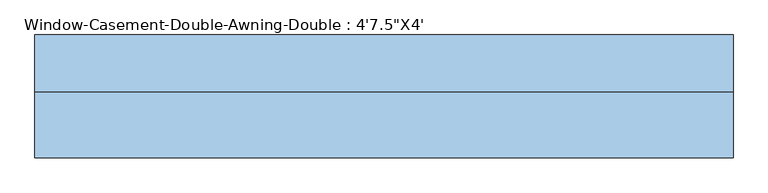
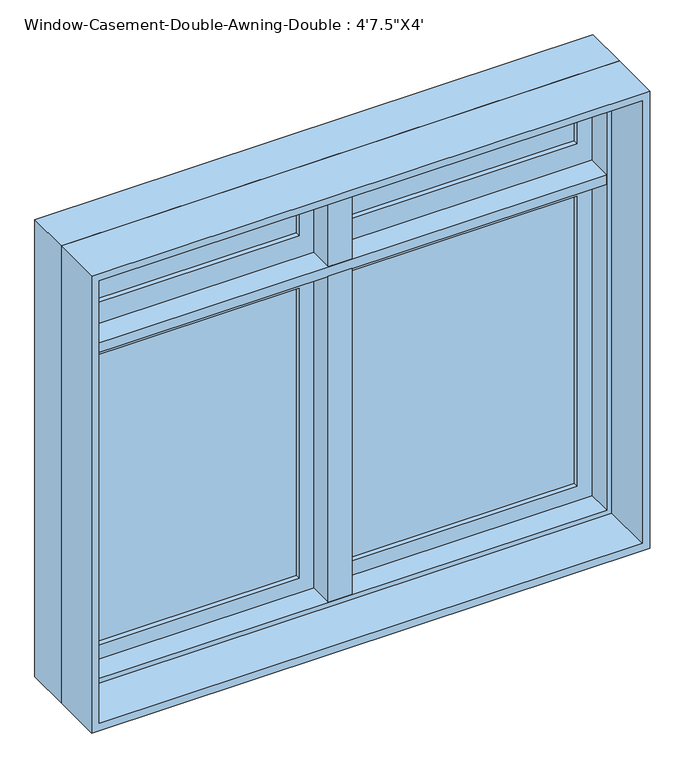
"""IFC4 building model written with IfcOpenShell, lengths in millimetres: window geometry."""

from ifc_helpers import new_model, si_unit, frame, origin, place, context, project, spatial, polyline, outline, extrude, faceted_brep, source, transform, mapped, element, save


def window_c5cb33f6(model_context):
    return source(origin(), model_context, "Body", "SolidModel", [
        faceted_brep([(673.1, 82.55, 2101.85), (673.1, 19.05, 2101.85), (-673.1, 19.05, 2101.85), (-673.1, 82.55, 2101.85), (692.15, 133.35, 2120.9), (692.15, 82.55, 2120.9), (-692.15, 82.55, 2120.9), (-692.15, 133.35, 2120.9), (704.85, 19.05, 2133.6), (704.85, 133.35, 2133.6), (-704.85, 133.35, 2133.6), (-704.85, 19.05, 2133.6), (-673.1, 19.05, 946.15), (-673.1, 82.55, 946.15), (-692.15, 82.55, 927.1), (-692.15, 133.35, 927.1), (-704.85, 133.35, 914.4), (-704.85, 19.05, 914.4), (673.1, 19.05, 946.15), (673.1, 82.55, 946.15), (692.15, 82.55, 927.1), (692.15, 133.35, 927.1), (704.85, 133.35, 914.4), (704.85, 19.05, 914.4)], [[[0, 1, 2, 3]], [[4, 5, 6, 7]], [[8, 9, 10, 11]], [[3, 2, 12, 13]], [[7, 6, 14, 15]], [[11, 10, 16, 17]], [[13, 12, 18, 19]], [[15, 14, 20, 21]], [[17, 16, 22, 23]], [[11, 17, 23, 8], [1, 18, 12, 2]], [[19, 18, 1, 0]], [[5, 20, 14, 6], [3, 13, 19, 0]], [[21, 20, 5, 4]], [[23, 22, 9, 8]], [[9, 22, 16, 10], [7, 15, 21, 4]]]),
        extrude(outline(polyline([(2133.6, -704.85), (914.4, -704.85), (914.4, 704.85), (2133.6, 704.85), (2133.6, -704.85)]), holes=[polyline([(2114.55, 685.8), (933.45, 685.8), (933.45, -685.8), (2114.55, -685.8), (2114.55, 685.8)])]), frame((0.0, -114.3, 0.0), z_axis=(0.0, 1.0, 0.0), x_axis=(0.0, 0.0, 1.0)), (0.0, 0.0, 1.0), 133.35),
        extrude(outline(polyline([(927.1, 692.15), (1816.1, 692.15), (1816.1, 9.525), (927.1, 9.525), (927.1, 692.15)]), holes=[polyline([(984.25, 66.675), (1758.95, 66.675), (1758.95, 635.0), (984.25, 635.0), (984.25, 66.675)])]), frame((0.0, 82.55, 0.0), z_axis=(0.0, 1.0, 0.0), x_axis=(0.0, 0.0, 1.0)), (0.0, 0.0, 1.0), 44.45),
        extrude(outline(polyline([(1816.1, -692.15), (927.1, -692.15), (927.1, -9.525), (1816.1, -9.525), (1816.1, -692.15)]), holes=[polyline([(1758.95, -66.675), (984.25, -66.675), (984.25, -635.0), (1758.95, -635.0), (1758.95, -66.675)])]), frame((0.0, 82.55, 0.0), z_axis=(0.0, 1.0, 0.0), x_axis=(0.0, 0.0, 1.0)), (0.0, 0.0, 1.0), 44.45),
        extrude(outline(polyline([(635.0, 114.3), (635.0, 107.95), (66.675, 107.95), (66.675, 114.3), (635.0, 114.3)])), frame((0.0, 0.0, 984.25), z_axis=(0.0, 0.0, 1.0), x_axis=(1.0, 0.0, 0.0)), (0.0, 0.0, 1.0), 774.7),
        extrude(outline(polyline([(66.675, 95.25), (66.675, 101.6), (635.0, 101.6), (635.0, 95.25), (66.675, 95.25)])), frame((0.0, 0.0, 984.25), z_axis=(0.0, 0.0, 1.0), x_axis=(1.0, 0.0, 0.0)), (0.0, 0.0, 1.0), 774.7),
        extrude(outline(polyline([(-66.675, 114.3), (-66.675, 107.95), (-635.0, 107.95), (-635.0, 114.3), (-66.675, 114.3)])), frame((0.0, 0.0, 984.25), z_axis=(0.0, 0.0, 1.0), x_axis=(1.0, 0.0, 0.0)), (0.0, 0.0, 1.0), 774.7),
        extrude(outline(polyline([(-635.0, 95.25), (-635.0, 101.6), (-66.675, 101.6), (-66.675, 95.25), (-635.0, 95.25)])), frame((0.0, 0.0, 984.25), z_axis=(0.0, 0.0, 1.0), x_axis=(1.0, 0.0, 0.0)), (0.0, 0.0, 1.0), 774.7),
        faceted_brep([(9.525, 133.35, 1816.1), (-9.525, 133.35, 1816.1), (-9.525, 82.55, 1816.1), (-30.1625, 82.55, 1816.1), (-30.1625, 19.05, 1816.1), (30.1625, 19.05, 1816.1), (30.1625, 82.55, 1816.1), (9.525, 82.55, 1816.1), (9.525, 133.35, 927.1), (9.525, 82.55, 927.1), (-9.525, 82.55, 927.1), (-9.525, 133.35, 927.1), (-9.525, 82.55, 946.15), (-30.1625, 82.55, 946.15), (-30.1625, 19.05, 946.15), (30.1625, 19.05, 946.15), (30.1625, 82.55, 946.15), (9.525, 82.55, 946.15)], [[[0, 1, 2, 3, 4, 5, 6, 7]], [[8, 9, 10, 11]], [[1, 0, 8, 11]], [[2, 1, 11, 10, 12]], [[3, 2, 12, 13]], [[4, 3, 13, 14]], [[5, 4, 14, 15]], [[6, 5, 15, 16]], [[7, 6, 16, 17]], [[0, 7, 17, 9, 8]], [[17, 12, 10, 9]], [[12, 17, 16, 15, 14, 13]]]),
        extrude(outline(polyline([(-66.675, 114.3), (-66.675, 107.95), (-635.0, 107.95), (-635.0, 114.3), (-66.675, 114.3)])), frame((0.0, 0.0, 1898.65), z_axis=(0.0, 0.0, 1.0), x_axis=(1.0, 0.0, 0.0)), (0.0, 0.0, 1.0), 165.1),
        extrude(outline(polyline([(-635.0, 95.25), (-635.0, 101.6), (-66.675, 101.6), (-66.675, 95.25), (-635.0, 95.25)])), frame((0.0, 0.0, 1898.65), z_axis=(0.0, 0.0, 1.0), x_axis=(1.0, 0.0, 0.0)), (0.0, 0.0, 1.0), 165.1),
        extrude(outline(polyline([(692.15, 133.35), (692.15, 82.55), (673.1, 82.55), (673.1, 19.05), (-673.1, 19.05), (-673.1, 82.55), (-692.15, 82.55), (-692.15, 133.35), (692.15, 133.35)])), frame((0.0, 0.0, 1816.1), z_axis=(0.0, 0.0, 1.0), x_axis=(1.0, 0.0, 0.0)), (0.0, 0.0, 1.0), 25.4),
        faceted_brep([(9.525, 82.55, 2120.9), (9.525, 133.35, 2120.9), (-9.525, 133.35, 2120.9), (-9.525, 82.55, 2120.9), (-9.525, 82.55, 1841.5), (-9.525, 133.35, 1841.5), (9.525, 133.35, 1841.5), (9.525, 82.55, 1841.5), (30.1625, 82.55, 1841.5), (30.1625, 19.05, 1841.5), (-30.1625, 19.05, 1841.5), (-30.1625, 82.55, 1841.5), (-30.1625, 82.55, 2101.85), (-9.525, 82.55, 2101.85), (-30.1625, 19.05, 2101.85), (30.1625, 19.05, 2101.85), (30.1625, 82.55, 2101.85), (9.525, 82.55, 2101.85)], [[[0, 1, 2, 3]], [[4, 5, 6, 7, 8, 9, 10, 11]], [[4, 11, 12, 13]], [[11, 10, 14, 12]], [[10, 9, 15, 14]], [[9, 8, 16, 15]], [[8, 7, 17, 16]], [[1, 0, 17, 7, 6]], [[2, 1, 6, 5]], [[3, 2, 5, 4, 13]], [[17, 13, 12, 14, 15, 16]], [[13, 17, 0, 3]]]),
        extrude(outline(polyline([(2120.9, 9.525), (1841.5, 9.525), (1841.5, 692.15), (2120.9, 692.15), (2120.9, 9.525)]), holes=[polyline([(2063.75, 635.0), (1898.65, 635.0), (1898.65, 66.675), (2063.75, 66.675), (2063.75, 635.0)])]), frame((0.0, 82.55, 0.0), z_axis=(0.0, 1.0, 0.0), x_axis=(0.0, 0.0, 1.0)), (0.0, 0.0, 1.0), 44.45),
        extrude(outline(polyline([(1841.5, -9.525), (2120.9, -9.525), (2120.9, -692.15), (1841.5, -692.15), (1841.5, -9.525)]), holes=[polyline([(1898.65, -635.0), (2063.75, -635.0), (2063.75, -66.675), (1898.65, -66.675), (1898.65, -635.0)])]), frame((0.0, 82.55, 0.0), z_axis=(0.0, 1.0, 0.0), x_axis=(0.0, 0.0, 1.0)), (0.0, 0.0, 1.0), 44.45),
        extrude(outline(polyline([(66.675, 114.3), (635.0, 114.3), (635.0, 107.95), (66.675, 107.95), (66.675, 114.3)])), frame((0.0, 0.0, 1898.65), z_axis=(0.0, 0.0, 1.0), x_axis=(1.0, 0.0, 0.0)), (0.0, 0.0, 1.0), 165.1),
        extrude(outline(polyline([(635.0, 95.25), (66.675, 95.25), (66.675, 101.6), (635.0, 101.6), (635.0, 95.25)])), frame((0.0, 0.0, 1898.65), z_axis=(0.0, 0.0, 1.0), x_axis=(1.0, 0.0, 0.0)), (0.0, 0.0, 1.0), 165.1),
    ])


if __name__ == "__main__":
    model = new_model("IFC4")
    model_context = context("Model", 3, world=origin())
    ifc_project = project(units=[si_unit("LENGTHUNIT", "METRE", prefix="MILLI")], contexts=[model_context])
    site = spatial("IfcSite", under=ifc_project)
    building = spatial("IfcBuilding", under=site)
    placement = place(None, origin())
    window_shape = window_c5cb33f6(model_context)
    element("IfcWindow", 1, ObjectType="Window-Casement-Double-Awning-Double : 4'7.5\"X4'", at=placement, inside=building, context=model_context, shape_type="MappedRepresentation", body=[
        mapped(window_shape, transform((0.0, 0.0, 0.0), x_axis=(1.0, 0.0, 0.0), y_axis=(0.0, 1.0, 0.0), z_axis=(0.0, 0.0, 1.0))),
    ])
    save(model, "model.ifc")

# Revit data of these elements
# Type "Window-Casement-Double-Awning-Double : 4'7.5\"X4'"
#   Type Mark = "21"
#   Fire Rating = "0.5h"
#   Assembly Code = "B2020100"
#   Analytic Construction = "Double glazing - domestic"
#   Window Inset [instance default] = 0' - 0"
#   Wall Thickness [instance default] = 0' - 6"
#   Interior Wall Closure [instance default] = 0' - 2 1/4"
#   Half Width = 2' - 3 3/4"
#   Visual Light Transmittance = 0.81
#   Transom Height = 1' - 0"
#   Thermal Resistance (R) = 1.8146 (h·ft²·°F)/BTU
#   Solar Heat Gain Coefficient = 0.76
#   Rough Width = 4' - 8"
#   Rough Height = 4' - 0 1/2"
#   Open Window Height = 3' - 0"
#   Frame Extension [instance default] = 0' - 0 1/4"
#   Height = 4' - 0"
#   Heat Transfer Coefficient (U) = 0.5511 BTU/(h·ft²·°F)
#   Exterior Wall Closure [instance default] = 0' - 1 1/4"
#   Extension Jamb [instance default] = 0' - 2 1/4"
#   Default Sill Height = 3' - 0"
#   Width = 4' - 7 1/2"
#   Top Muntin Visibility = yes
#   Bottom Muntin Visibility = yes
#   Interior Trim Visibility [instance default] = yes
#   Exterior Trim Visibility [instance default] = yes
#   Extension Jamb Visibility [instance default] = yes
#   Interior Trim Material = Wood - Stained
#   Muntin Pattern = Muntin Pattern_2x2 : Muntin Pattern_2x2
#   Interior Trim = Trim-Window-Interior-Flat : Picture Frame
#   Interior Frame Material = Wood - Stained
#   Glass Panel Material = Glass
#   Exterior Trim Material = Clad - White
#   Exterior Trim = Trim-Window-Exterior-Flat : with Sill
#   Exterior Frame Material = Clad - White
#   Wall Closure = (empty or 0)
# Element 1 (IfcWindow, "Window-Casement-Double-Awning-Double : 4'7.5\"X4'")
#   Wall Thickness = 0' - 9"
#   Extension Jamb = 0' - 5 1/4"
#   Materials on its faces: "Wood - Stained", "Glass", "Clad - White"
# Materials
#   "Wood - Stained": class "Wood", colour RGB 224 178 126, transparency 0, Cost = 0
#   "Glass": class "Glass", colour RGB 0 128 192, transparency 0.75, Description = "Soda Lime Glass", Cost = 0
#   "Clad - White": class "Wood", colour RGB 242 242 238, transparency 0, Cost = 0
